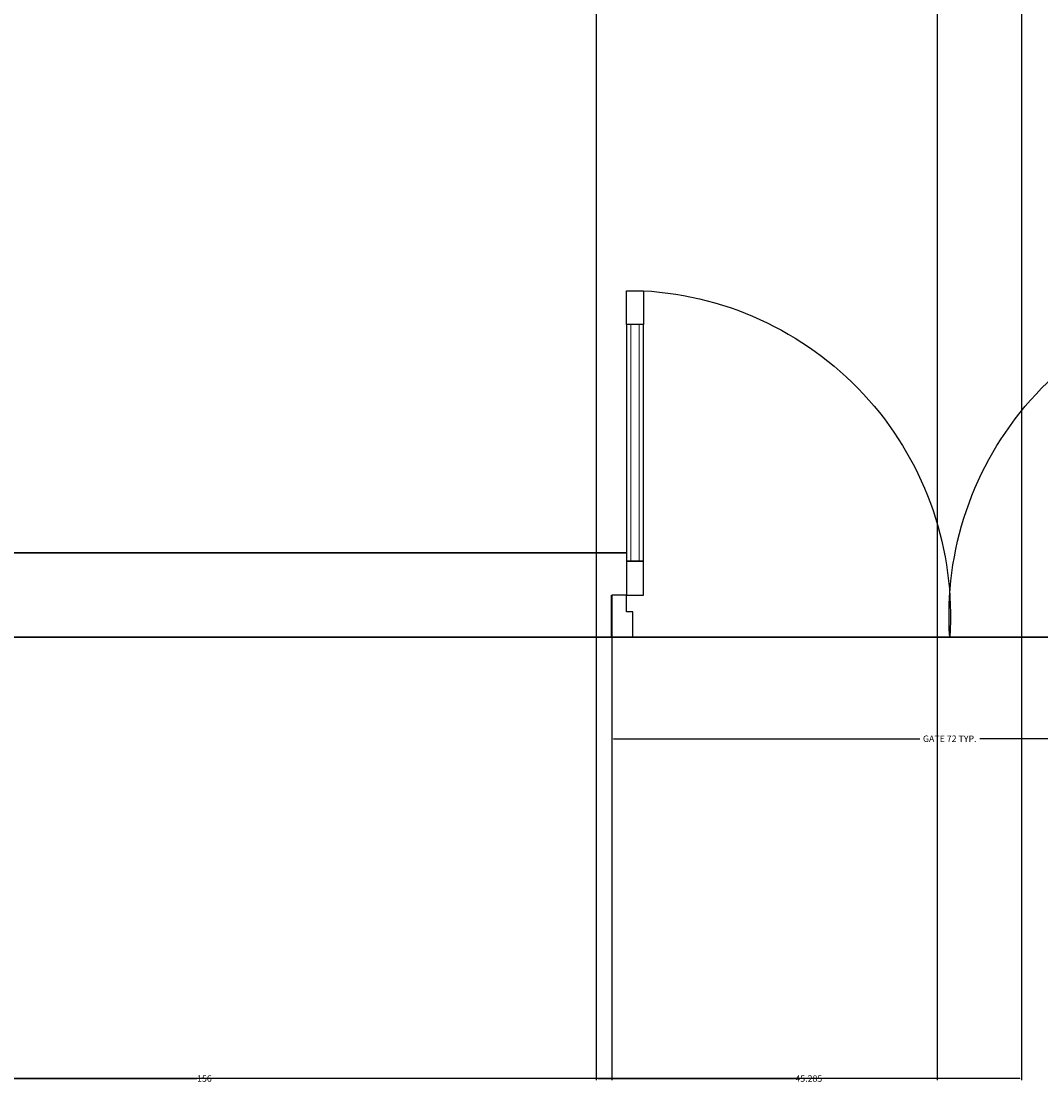
# Model space of a CAD drawing. Units: inches. Extents: x 867 to 1667, y -234 to 788.
# Tile 19 of 42: x 1462 to 1571, y -234 to -121. Entities that reach past the tile are written whole.
import ezdxf

# ---------------------------------------------------------------- set-up
doc = ezdxf.new("R2010")
doc.units = ezdxf.units.IN
doc.header["$MEASUREMENT"] = 0
for name, color, linetype, lineweight in [('A-ANNO-DIMS', 2, 'Continuous', 18), ('A-Door', 150, 'Continuous', 25), ('A-Glaz', 92, 'Continuous', 18), ('A-Wall', 7, 'Continuous', 35), ('A-WALL-SITE', 8, 'Continuous', 30)]:
    doc.layers.add(name, color=color, linetype=linetype, lineweight=lineweight)
doc.layers.add('NT', color=1, linetype='Continuous')
doc.styles.get("Standard").update_dxf_attribs({"font": 'arial.ttf'})
doc.dimstyles.get("Standard").update_dxf_attribs({"dimtxt": 0.6875, "dimasz": 0.18, "dimexe": 0.18, "dimexo": 0.0625, "dimgap": 0.09, "dimtad": 0, "dimdec": 4, "dimzin": 0, "dimdsep": 46, "dimlunit": 4, "dimtxsty": 'Standard', "dimcen": 0.09, "dimadec": 0, "dimazin": 0, "dimtfac": 1, "dimtdec": 4, "dimtofl": 0, "dimtmove": 0, "dimatfit": 3, "dimfxl": 1, "dimtolj": 1, "dimtzin": 0, "dimarcsym": 0})

# ---------------------------------------------------------------- blocks, each defined once
blk = doc.blocks.new('A$C0EE93B68')
at = {"layer": 'A-Door'}
for points in [[(100, 1565), (100, 1600), (0, 1600), (0, 1550), (50, 1550), (60, 1550), (60, 1565)], [(100, 1525), (180, 1525), (180, 1565), (100, 1565)], [(180, 1525), (740, 1525), (740, 1565), (180, 1565)], [(820, 1525), (740, 1525), (740, 1565), (820, 1565)], [(100, 75), (180, 75), (180, 35), (100, 35)], [(180, 75), (740, 75), (740, 35), (180, 35)], [(820, 75), (740, 75), (740, 35), (820, 35)], [(100, 35), (100, 0), (0, 0), (0, 50), (50, 50), (60, 50), (60, 35)]]:
    blk.add_lwpolyline(points, close=True, dxfattribs=at)
at = {"layer": 'A-Glaz'}
for points in [[(180, 1535), (740, 1535), (740, 1555), (180, 1555)], [(180, 65), (740, 65), (740, 45), (180, 45)]]:
    blk.add_lwpolyline(points, close=True, dxfattribs=at)
at = {"layer": 'A-Wall'}
for p, q in [((0, 1600), (100, 1600)), ((0, 0), (100, 0))]:
    blk.add_line(p, q, dxfattribs=at)
at = {"layer": 'NT'}
for centre, start, end in [((51.6, 1567.9), 266.1547, 356.8081), ((51.6, 32.1), 3.1919, 93.8453)]:
    blk.add_arc(centre, 769.6, start, end, dxfattribs=at)
blk = doc.blocks.new('*D9')
at = {"layer": 'A-ANNO-DIMS', "color": 0, "lineweight": -2, "transparency": 16777216}
for p, q in [((1525.26, -186.47), (1525.26, -197.38)), ((1597.22, -186.47), (1597.22, -197.38)), ((1525.44, -197.2), (1558.05, -197.2)), ((1597.04, -197.2), (1564.44, -197.2))]:
    blk.add_line(p, q, dxfattribs=at)
at = {"layer": 'A-ANNO-DIMS', "color": 0, "transparency": 16777216}
for points in [[(1525.44, -197.17), (1525.44, -197.23), (1525.26, -197.2)], [(1597.04, -197.17), (1597.04, -197.23), (1597.22, -197.2)]]:
    blk.add_solid(points, dxfattribs=at)
at = {"layer": 'Defpoints', "color": 0, "transparency": 16777216}
for p in [(1525.26, -186.41), (1597.22, -186.41), (1597.22, -197.2)]:
    blk.add_point(p, dxfattribs=at)
at = {"layer": 'A-ANNO-DIMS', "color": 0, "transparency": 16777216, "insert": (1561.24, -197.2), "char_height": 0.6875, "attachment_point": 5}
blk.add_mtext('\\A1;GATE 72 TYP.', dxfattribs=at)
blk = doc.blocks.new('*D27')
at = {"layer": 'A-ANNO-DIMS', "color": 0, "lineweight": -2, "transparency": 16777216}
for p, q in [((1070.89, -55.97), (1070.89, -233.54)), ((1525.26, -186.47), (1525.26, -233.54)), ((1071.07, -233.36), (1296.81, -233.36)), ((1525.08, -233.36), (1299.34, -233.36))]:
    blk.add_line(p, q, dxfattribs=at)
at = {"layer": 'A-ANNO-DIMS', "color": 0, "transparency": 16777216}
for points in [[(1071.07, -233.33), (1071.07, -233.39), (1070.89, -233.36)], [(1525.08, -233.33), (1525.08, -233.39), (1525.26, -233.36)]]:
    blk.add_solid(points, dxfattribs=at)
at = {"layer": 'Defpoints', "color": 0, "transparency": 16777216}
for p in [(1070.89, -55.91), (1525.26, -186.41), (1525.26, -233.36)]:
    blk.add_point(p, dxfattribs=at)
at = {"layer": 'A-ANNO-DIMS', "color": 0, "transparency": 16777216, "insert": (1298.08, -233.36), "char_height": 0.688, "attachment_point": 5}
blk.add_mtext('\\A1;454.4', dxfattribs=at)
blk = doc.blocks.new('*D38')
at = {"layer": 'A-ANNO-DIMS', "color": 0, "lineweight": -2, "transparency": 16777216}
for p, q in [((1403.89, -7.95), (1403.89, -233.54)), ((1559.89, -7.95), (1559.89, -233.54)), ((1404.07, -233.36), (1481.07, -233.36)), ((1559.71, -233.36), (1482.7, -233.36))]:
    blk.add_line(p, q, dxfattribs=at)
at = {"layer": 'A-ANNO-DIMS', "color": 0, "transparency": 16777216}
for points in [[(1404.07, -233.33), (1404.07, -233.39), (1403.89, -233.36)], [(1559.71, -233.33), (1559.71, -233.39), (1559.89, -233.36)]]:
    blk.add_solid(points, dxfattribs=at)
at = {"layer": 'Defpoints', "color": 0, "transparency": 16777216}
for p in [(1403.89, -7.88), (1559.89, -7.88), (1559.89, -233.36)]:
    blk.add_point(p, dxfattribs=at)
at = {"layer": 'A-ANNO-DIMS', "color": 0, "transparency": 16777216, "insert": (1481.89, -233.36), "char_height": 0.688, "attachment_point": 5}
blk.add_mtext('\\A1;156', dxfattribs=at)
blk = doc.blocks.new('*D55')
at = {"layer": 'A-ANNO-DIMS', "color": 0, "lineweight": -2, "transparency": 16777216}
for p, q in [((1523.6, 257.55), (1523.6, -233.54)), ((1568.89, 257.55), (1568.89, -233.54)), ((1523.78, -233.36), (1544.71, -233.36)), ((1568.71, -233.36), (1547.78, -233.36))]:
    blk.add_line(p, q, dxfattribs=at)
at = {"layer": 'A-ANNO-DIMS', "color": 0, "transparency": 16777216}
for points in [[(1523.78, -233.33), (1523.78, -233.39), (1523.6, -233.36)], [(1568.71, -233.33), (1568.71, -233.39), (1568.89, -233.36)]]:
    blk.add_solid(points, dxfattribs=at)
at = {"layer": 'Defpoints', "color": 0, "transparency": 16777216}
for p in [(1523.6, 257.62), (1568.89, 257.62), (1568.89, -233.36)]:
    blk.add_point(p, dxfattribs=at)
at = {"layer": 'A-ANNO-DIMS', "color": 0, "transparency": 16777216, "insert": (1546.24, -233.36), "char_height": 0.688, "attachment_point": 5}
blk.add_mtext('\\A1;45.285', dxfattribs=at)

msp = doc.modelspace()

# ---------------------------------------------------------------- linework, layer by layer
at = {"layer": 'A-WALL-SITE'}
for p, q in [((1526.8389, -177.4081), (1006.3882, -177.4081)), ((1619.8866, -186.4081), (914.8866, -186.4081))]:
    msp.add_line(p, q, dxfattribs=at)

# ---------------------------------------------------------------- block references
at = {"layer": 'A-Door', "xscale": -0.0449743717352066, "yscale": 0.0449743717352066, "zscale": 0.0449743717352066, "rotation": 270}
msp.add_blockref('A$C0EE93B68', (1525.2648, -186.4081), dxfattribs=at)

# ---------------------------------------------------------------- dimensions: what is measured, and where the dimension line sits
at = {"layer": 'A-ANNO-DIMS'}
for base, p1, p2, override, picture, middle in [((1568.8866, -233.3581), (1523.6015, 257.617), (1568.8866, 257.617), {"dimdec": 3, "dimlfac": 1, "dimrnd": 0, "dimzin": 0, "dimdsep": 46, "dimlunit": 2}, '*D55', (1546.2441, -233.3581)), ((1559.8866, -233.3581), (1403.8866, -7.883), (1559.8866, -7.883), {"dimdec": 0, "dimlfac": 1, "dimrnd": 0, "dimzin": 0, "dimdsep": 46, "dimlunit": 2}, '*D38', (1481.8866, -233.3581)), ((1525.2648, -233.3581), (1070.8866, -55.9081), (1525.2648, -186.4081), {"dimdec": 1, "dimlfac": 1, "dimrnd": 0, "dimzin": 0, "dimdsep": 46, "dimlunit": 2}, '*D27', (1298.0757, -233.3581))]:
    dim = msp.add_linear_dim(base=base, p1=p1, p2=p2, dimstyle='Standard', override=override, dxfattribs=at)
    dim.commit()
    dim.dimension.update_dxf_attribs({"geometry": picture, "text_midpoint": middle})
dim = msp.add_linear_dim(base=(1597.2238, -197.2019), p1=(1525.2648, -186.4081), p2=(1597.2238, -186.4081), text='GATE <> TYP.', dimstyle='Standard', override={"dimdec": 0, "dimlfac": 1, "dimrnd": 0, "dimzin": 0, "dimdsep": 46, "dimlunit": 2}, dxfattribs=at)
dim.commit()
dim.dimension.update_dxf_attribs({"geometry": '*D9', "text_midpoint": (1561.2443, -197.2019)})

doc.saveas('drawing.dxf')
